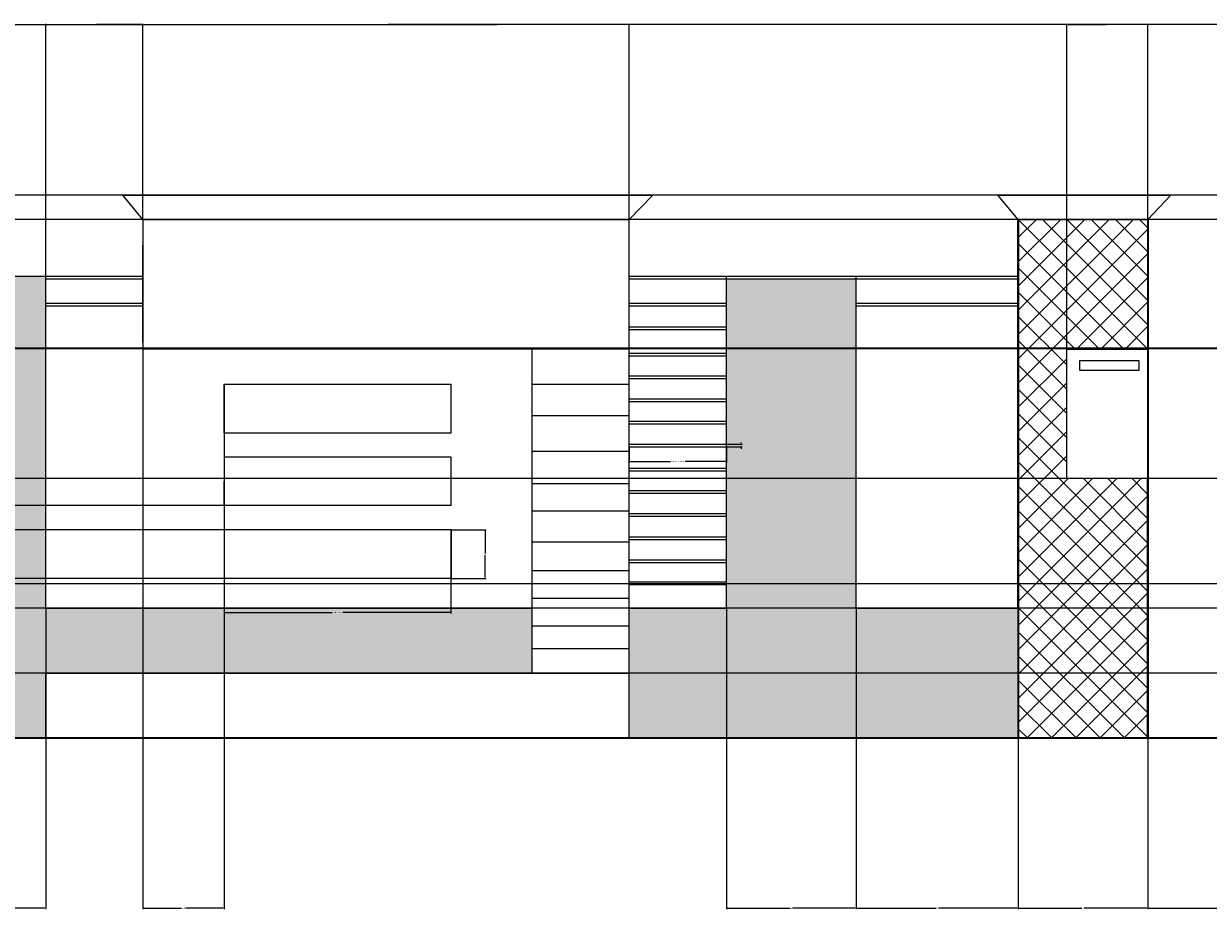
# Model space of a CAD drawing. Units: inches. Extents: x 2121 to 2815, y 1818 to 2233.
# Tile 2 of 6: x 2311 to 2530, y 1818 to 1982. Entities that reach past the tile are written whole.
import ezdxf

# ---------------------------------------------------------------- set-up
doc = ezdxf.new("R2010")
doc.units = ezdxf.units.IN
for name, color, linetype, lineweight in [('A-ANNO-DIMS', 2, 'Continuous', 18), ('A-COLS', 7, 'Continuous', 35), ('A-DETL', 7, 'Continuous', 18), ('A-ELEV', 7, 'Continuous', 25), ('A-ELEV-GRDE', 7, 'Continuous', 35), ('A-ELEV-SLAT', 7, 'Continuous', 18), ('A-WALL-COPG', 7, 'Continuous', 25), ('A-WALL-PATT', 8, 'Continuous', 13)]:
    doc.layers.add(name, color=color, linetype=linetype, lineweight=lineweight)
doc.styles.get("Standard").update_dxf_attribs({"font": 'arial.ttf'})
doc.dimstyles.get("Standard").update_dxf_attribs({"dimtxt": 0.18, "dimasz": 0.18, "dimexe": 0.18, "dimexo": 0.0625, "dimgap": 0.09, "dimtad": 0, "dimtih": 1, "dimtoh": 1, "dimdec": 4, "dimzin": 0, "dimdsep": 46, "dimtxsty": 'Standard', "dimcen": 0.09, "dimadec": 0, "dimazin": 0, "dimtfac": 1, "dimtdec": 4, "dimtofl": 0, "dimtmove": 0, "dimatfit": 3, "dimfxl": 1, "dimtolj": 1, "dimtzin": 0, "dimarcsym": 0})

# ---------------------------------------------------------------- blocks, each defined once
blk = doc.blocks.new('WALL-SLAT-18')
for p, q in [((0, 0.5), (18, 0.5)), ((0, 0), (18, 0)), ((0, 0), (18, 0))]:
    blk.add_line(p, q)
blk = doc.blocks.new('WALL-PANEL-42X9')
for p, q in [((42, 9), (0, 9)), ((0, 9), (0, 0)), ((42, 0), (42, 9)), ((42, 0), (0, 0))]:
    blk.add_line(p, q)
blk = doc.blocks.new('*D4')
at = {"layer": 'A-ANNO-DIMS', "color": 0, "lineweight": -2, "transparency": 16777216}
for p, q in [((2422.83, 1903.71), (2422.83, 1900.89)), ((2440.83, 1903.71), (2440.83, 1900.89)), ((2423.01, 1901.07), (2430.48, 1901.07)), ((2440.65, 1901.07), (2433.18, 1901.07))]:
    blk.add_line(p, q, dxfattribs=at)
at = {"layer": 'A-ANNO-DIMS', "color": 0, "transparency": 16777216}
for points in [[(2423.01, 1901.1), (2423.01, 1901.04), (2422.83, 1901.07)], [(2440.65, 1901.1), (2440.65, 1901.04), (2440.83, 1901.07)]]:
    blk.add_solid(points, dxfattribs=at)
at = {"layer": 'Defpoints', "color": 0, "transparency": 16777216}
for p in [(2422.83, 1903.77), (2440.83, 1903.77), (2440.83, 1901.07)]:
    blk.add_point(p, dxfattribs=at)
at = {"layer": 'A-ANNO-DIMS', "color": 0, "transparency": 16777216, "insert": (2431.83, 1901.07), "char_height": 0.18, "attachment_point": 5}
blk.add_mtext('\\A1;SHORT SLAT 18 TYP.', dxfattribs=at)
blk = doc.blocks.new('*D5')
at = {"layer": 'A-ANNO-DIMS', "color": 0, "lineweight": -2, "transparency": 16777216}
for p, q in [((2440.9, 1904.27), (2443.71, 1904.27)), ((2440.9, 1903.77), (2443.71, 1903.77)), ((2443.53, 1904.45), (2443.53, 1904.63)), ((2443.53, 1903.59), (2443.53, 1903.41))]:
    blk.add_line(p, q, dxfattribs=at)
at = {"layer": 'A-ANNO-DIMS', "color": 0, "transparency": 16777216}
for points in [[(2443.5, 1904.45), (2443.56, 1904.45), (2443.53, 1904.27)], [(2443.5, 1903.59), (2443.56, 1903.59), (2443.53, 1903.77)]]:
    blk.add_solid(points, dxfattribs=at)
at = {"layer": 'Defpoints', "color": 0, "transparency": 16777216}
for p in [(2440.83, 1904.27), (2440.83, 1903.77), (2443.53, 1904.27)]:
    blk.add_point(p, dxfattribs=at)
at = {"layer": 'A-ANNO-DIMS', "color": 0, "transparency": 16777216, "insert": (2443.53, 1904.02), "char_height": 0.18, "attachment_point": 5}
blk.add_mtext('\\A1;1 TYP.', dxfattribs=at)
blk = doc.blocks.new('*D6')
at = {"layer": 'A-ANNO-DIMS', "color": 0, "lineweight": -2, "transparency": 16777216}
for p, q in [((2347.83, 1879.34), (2347.83, 1872.93)), ((2389.83, 1879.34), (2389.83, 1872.93)), ((2348.01, 1873.11), (2367.86, 1873.11)), ((2389.65, 1873.11), (2369.8, 1873.11))]:
    blk.add_line(p, q, dxfattribs=at)
at = {"layer": 'A-ANNO-DIMS', "color": 0, "transparency": 16777216}
for points in [[(2348.01, 1873.14), (2348.01, 1873.08), (2347.83, 1873.11)], [(2389.65, 1873.14), (2389.65, 1873.08), (2389.83, 1873.11)]]:
    blk.add_solid(points, dxfattribs=at)
at = {"layer": 'Defpoints', "color": 0, "transparency": 16777216}
for p in [(2347.83, 1879.41), (2389.83, 1879.41), (2389.83, 1873.11)]:
    blk.add_point(p, dxfattribs=at)
at = {"layer": 'A-ANNO-DIMS', "color": 0, "transparency": 16777216, "insert": (2368.83, 1873.11), "char_height": 0.18, "attachment_point": 5}
blk.add_mtext('\\A1;PANEL 42 TYP.', dxfattribs=at)
blk = doc.blocks.new('*D7')
at = {"layer": 'A-ANNO-DIMS', "color": 0, "lineweight": -2, "transparency": 16777216}
for p, q in [((2389.9, 1888.41), (2396.31, 1888.41)), ((2396.13, 1888.23), (2396.13, 1884.09)), ((2396.13, 1879.59), (2396.13, 1883.73)), ((2389.9, 1879.41), (2396.31, 1879.41))]:
    blk.add_line(p, q, dxfattribs=at)
at = {"layer": 'A-ANNO-DIMS', "color": 0, "transparency": 16777216}
for points in [[(2396.1, 1888.23), (2396.16, 1888.23), (2396.13, 1888.41)], [(2396.1, 1879.59), (2396.16, 1879.59), (2396.13, 1879.41)]]:
    blk.add_solid(points, dxfattribs=at)
at = {"layer": 'Defpoints', "color": 0, "transparency": 16777216}
for p in [(2389.83, 1888.41), (2396.13, 1888.41), (2389.83, 1879.41)]:
    blk.add_point(p, dxfattribs=at)
at = {"layer": 'A-ANNO-DIMS', "color": 0, "transparency": 16777216, "insert": (2396.13, 1883.91), "char_height": 0.18, "attachment_point": 5}
blk.add_mtext('\\A1;9 TYP.', dxfattribs=at)
blk = doc.blocks.new('*D43')
at = {"layer": 'A-ANNO-DIMS', "color": 0, "lineweight": -2, "transparency": 16777216}
for p, q in [((2152.83, 1935.47), (2152.83, 1982.13)), ((2644.63, 1950.47), (2644.63, 1982.13)), ((2153.01, 1981.95), (2398.33, 1981.95)), ((2644.45, 1981.95), (2399.13, 1981.95))]:
    blk.add_line(p, q, dxfattribs=at)
at = {"layer": 'A-ANNO-DIMS', "color": 0, "transparency": 16777216}
for points in [[(2153.01, 1981.98), (2153.01, 1981.92), (2152.83, 1981.95)], [(2644.45, 1981.98), (2644.45, 1981.92), (2644.63, 1981.95)]]:
    blk.add_solid(points, dxfattribs=at)
at = {"layer": 'Defpoints', "color": 0, "transparency": 16777216}
for p in [(2644.63, 1981.95), (2644.63, 1950.41), (2152.83, 1935.41)]:
    blk.add_point(p, dxfattribs=at)
at = {"layer": 'A-ANNO-DIMS', "color": 0, "transparency": 16777216, "insert": (2398.73, 1981.95), "char_height": 0.18, "attachment_point": 5}
blk.add_mtext('\\A1;491.8', dxfattribs=at)
blk = doc.blocks.new('*D51')
at = {"layer": 'A-ANNO-DIMS', "color": 0, "lineweight": -2, "transparency": 16777216}
for p, q in [((2290.83, 1873.84), (2290.83, 1818.19)), ((2314.83, 1873.84), (2314.83, 1818.19)), ((2291.01, 1818.37), (2302.61, 1818.37)), ((2314.65, 1818.37), (2303.05, 1818.37))]:
    blk.add_line(p, q, dxfattribs=at)
at = {"layer": 'A-ANNO-DIMS', "color": 0, "transparency": 16777216}
for points in [[(2291.01, 1818.4), (2291.01, 1818.34), (2290.83, 1818.37)], [(2314.65, 1818.4), (2314.65, 1818.34), (2314.83, 1818.37)]]:
    blk.add_solid(points, dxfattribs=at)
at = {"layer": 'Defpoints', "color": 0, "transparency": 16777216}
for p in [(2290.83, 1873.91), (2314.83, 1873.91), (2314.83, 1818.37)]:
    blk.add_point(p, dxfattribs=at)
at = {"layer": 'A-ANNO-DIMS', "color": 0, "transparency": 16777216, "insert": (2302.83, 1818.37), "char_height": 0.18, "attachment_point": 5}
blk.add_mtext('\\A1;24', dxfattribs=at)
blk = doc.blocks.new('*D52')
at = {"layer": 'A-ANNO-DIMS', "color": 0, "lineweight": -2, "transparency": 16777216}
for p, q in [((2314.83, 1935.47), (2314.83, 1982.13)), ((2332.79, 1945.97), (2332.79, 1982.13)), ((2315.01, 1981.95), (2323.43, 1981.95)), ((2332.61, 1981.95), (2324.2, 1981.95))]:
    blk.add_line(p, q, dxfattribs=at)
at = {"layer": 'A-ANNO-DIMS', "color": 0, "transparency": 16777216}
for points in [[(2315.01, 1981.98), (2315.01, 1981.92), (2314.83, 1981.95)], [(2332.61, 1981.98), (2332.61, 1981.92), (2332.79, 1981.95)]]:
    blk.add_solid(points, dxfattribs=at)
at = {"layer": 'Defpoints', "color": 0, "transparency": 16777216}
for p in [(2332.79, 1981.95), (2332.79, 1945.91), (2314.83, 1935.41)]:
    blk.add_point(p, dxfattribs=at)
at = {"layer": 'A-ANNO-DIMS', "color": 0, "transparency": 16777216, "insert": (2323.81, 1981.95), "char_height": 0.18, "attachment_point": 5}
blk.add_mtext('\\A1;17.96', dxfattribs=at)
blk = doc.blocks.new('*D53')
at = {"layer": 'A-ANNO-DIMS', "color": 0, "lineweight": -2, "transparency": 16777216}
for p, q in [((2332.79, 1945.97), (2332.79, 1982.13)), ((2422.83, 1945.97), (2422.83, 1982.13)), ((2332.97, 1981.95), (2377.42, 1981.95)), ((2422.65, 1981.95), (2378.21, 1981.95))]:
    blk.add_line(p, q, dxfattribs=at)
at = {"layer": 'A-ANNO-DIMS', "color": 0, "transparency": 16777216}
for points in [[(2332.97, 1981.98), (2332.97, 1981.92), (2332.79, 1981.95)], [(2422.65, 1981.98), (2422.65, 1981.92), (2422.83, 1981.95)]]:
    blk.add_solid(points, dxfattribs=at)
at = {"layer": 'Defpoints', "color": 0, "transparency": 16777216}
for p in [(2422.83, 1981.95), (2332.79, 1945.91), (2422.83, 1945.91)]:
    blk.add_point(p, dxfattribs=at)
at = {"layer": 'A-ANNO-DIMS', "color": 0, "transparency": 16777216, "insert": (2377.81, 1981.95), "char_height": 0.18, "attachment_point": 5}
blk.add_mtext('\\A1;90.04', dxfattribs=at)
blk = doc.blocks.new('*D54')
at = {"layer": 'A-ANNO-DIMS', "color": 0, "lineweight": -2, "transparency": 16777216}
for p, q in [((2440.83, 1873.84), (2440.83, 1818.19)), ((2464.83, 1873.84), (2464.83, 1818.19)), ((2441.01, 1818.37), (2452.61, 1818.37)), ((2464.65, 1818.37), (2453.05, 1818.37))]:
    blk.add_line(p, q, dxfattribs=at)
at = {"layer": 'A-ANNO-DIMS', "color": 0, "transparency": 16777216}
for points in [[(2441.01, 1818.4), (2441.01, 1818.34), (2440.83, 1818.37)], [(2464.65, 1818.4), (2464.65, 1818.34), (2464.83, 1818.37)]]:
    blk.add_solid(points, dxfattribs=at)
at = {"layer": 'Defpoints', "color": 0, "transparency": 16777216}
for p in [(2440.83, 1873.91), (2464.83, 1873.91), (2464.83, 1818.37)]:
    blk.add_point(p, dxfattribs=at)
at = {"layer": 'A-ANNO-DIMS', "color": 0, "transparency": 16777216, "insert": (2452.83, 1818.37), "char_height": 0.18, "attachment_point": 5}
blk.add_mtext('\\A1;24', dxfattribs=at)
blk = doc.blocks.new('*D55')
at = {"layer": 'A-ANNO-DIMS', "color": 0, "lineweight": -2, "transparency": 16777216}
for p, q in [((2464.83, 1873.84), (2464.83, 1818.19)), ((2494.83, 1873.84), (2494.83, 1818.19)), ((2465.01, 1818.37), (2479.61, 1818.37)), ((2494.65, 1818.37), (2480.05, 1818.37))]:
    blk.add_line(p, q, dxfattribs=at)
at = {"layer": 'A-ANNO-DIMS', "color": 0, "transparency": 16777216}
for points in [[(2465.01, 1818.4), (2465.01, 1818.34), (2464.83, 1818.37)], [(2494.65, 1818.4), (2494.65, 1818.34), (2494.83, 1818.37)]]:
    blk.add_solid(points, dxfattribs=at)
at = {"layer": 'Defpoints', "color": 0, "transparency": 16777216}
for p in [(2464.83, 1873.91), (2494.83, 1873.91), (2494.83, 1818.37)]:
    blk.add_point(p, dxfattribs=at)
at = {"layer": 'A-ANNO-DIMS', "color": 0, "transparency": 16777216, "insert": (2479.83, 1818.37), "char_height": 0.18, "attachment_point": 5}
blk.add_mtext('\\A1;30', dxfattribs=at)
blk = doc.blocks.new('*D56')
at = {"layer": 'A-ANNO-DIMS', "color": 0, "lineweight": -2, "transparency": 16777216}
for p, q in [((2494.83, 1849.84), (2494.83, 1818.19)), ((2518.83, 1849.84), (2518.83, 1818.19)), ((2495.01, 1818.37), (2506.61, 1818.37)), ((2518.65, 1818.37), (2507.05, 1818.37))]:
    blk.add_line(p, q, dxfattribs=at)
at = {"layer": 'A-ANNO-DIMS', "color": 0, "transparency": 16777216}
for points in [[(2495.01, 1818.4), (2495.01, 1818.34), (2494.83, 1818.37)], [(2518.65, 1818.4), (2518.65, 1818.34), (2518.83, 1818.37)]]:
    blk.add_solid(points, dxfattribs=at)
at = {"layer": 'Defpoints', "color": 0, "transparency": 16777216}
for p in [(2494.83, 1849.91), (2518.83, 1849.91), (2518.83, 1818.37)]:
    blk.add_point(p, dxfattribs=at)
at = {"layer": 'A-ANNO-DIMS', "color": 0, "transparency": 16777216, "insert": (2506.83, 1818.37), "char_height": 0.18, "attachment_point": 5}
blk.add_mtext('\\A1;24', dxfattribs=at)
blk = doc.blocks.new('*D57')
at = {"layer": 'A-ANNO-DIMS', "color": 0, "lineweight": -2, "transparency": 16777216}
for p, q in [((2518.83, 1849.84), (2518.83, 1818.19)), ((2619.83, 1849.84), (2619.83, 1818.19)), ((2519.01, 1818.37), (2569.07, 1818.37)), ((2619.65, 1818.37), (2569.6, 1818.37))]:
    blk.add_line(p, q, dxfattribs=at)
at = {"layer": 'A-ANNO-DIMS', "color": 0, "transparency": 16777216}
for points in [[(2519.01, 1818.4), (2519.01, 1818.34), (2518.83, 1818.37)], [(2619.65, 1818.4), (2619.65, 1818.34), (2619.83, 1818.37)]]:
    blk.add_solid(points, dxfattribs=at)
at = {"layer": 'Defpoints', "color": 0, "transparency": 16777216}
for p in [(2518.83, 1849.91), (2619.83, 1849.91), (2619.83, 1818.37)]:
    blk.add_point(p, dxfattribs=at)
at = {"layer": 'A-ANNO-DIMS', "color": 0, "transparency": 16777216, "insert": (2569.33, 1818.37), "char_height": 0.18, "attachment_point": 5}
blk.add_mtext('\\A1;101', dxfattribs=at)
blk = doc.blocks.new('*D59')
at = {"layer": 'A-ANNO-DIMS', "color": 0, "lineweight": -2, "transparency": 16777216}
for p, q in [((2182.9, 1922.1), (2815, 1922.1)), ((2814.82, 1921.92), (2814.82, 1886.18)), ((2814.82, 1850.09), (2814.82, 1885.82)), ((2182.9, 1849.91), (2815, 1849.91))]:
    blk.add_line(p, q, dxfattribs=at)
at = {"layer": 'A-ANNO-DIMS', "color": 0, "transparency": 16777216}
for points in [[(2814.79, 1921.92), (2814.85, 1921.92), (2814.82, 1922.1)], [(2814.79, 1850.09), (2814.85, 1850.09), (2814.82, 1849.91)]]:
    blk.add_solid(points, dxfattribs=at)
at = {"layer": 'Defpoints', "color": 0, "transparency": 16777216}
for p in [(2182.83, 1922.1), (2814.82, 1922.1), (2182.83, 1849.91)]:
    blk.add_point(p, dxfattribs=at)
at = {"layer": 'A-ANNO-DIMS', "color": 0, "transparency": 16777216, "insert": (2814.82, 1886), "char_height": 0.18, "attachment_point": 5}
blk.add_mtext('\\A1;72.2', dxfattribs=at)
blk = doc.blocks.new('*D61')
at = {"layer": 'A-ANNO-DIMS', "color": 0, "lineweight": -2, "transparency": 16777216}
for p, q in [((2314.77, 1861.91), (2121.11, 1861.91)), ((2121.29, 1861.73), (2121.29, 1856.09)), ((2121.29, 1850.09), (2121.29, 1855.73)), ((2314.77, 1849.91), (2121.11, 1849.91))]:
    blk.add_line(p, q, dxfattribs=at)
at = {"layer": 'A-ANNO-DIMS', "color": 0, "transparency": 16777216}
for points in [[(2121.26, 1861.73), (2121.32, 1861.73), (2121.29, 1861.91)], [(2121.26, 1850.09), (2121.32, 1850.09), (2121.29, 1849.91)]]:
    blk.add_solid(points, dxfattribs=at)
at = {"layer": 'Defpoints', "color": 0, "transparency": 16777216}
for p in [(2121.29, 1861.91), (2314.83, 1861.91), (2314.83, 1849.91)]:
    blk.add_point(p, dxfattribs=at)
at = {"layer": 'A-ANNO-DIMS', "color": 0, "transparency": 16777216, "insert": (2121.29, 1855.91), "char_height": 0.18, "attachment_point": 5}
blk.add_mtext('\\A1;12', dxfattribs=at)
blk = doc.blocks.new('*D62')
at = {"layer": 'A-ANNO-DIMS', "color": 0, "lineweight": -2, "transparency": 16777216}
for p, q in [((2332.79, 1921.84), (2332.79, 1818.19)), ((2347.83, 1915.34), (2347.83, 1818.19)), ((2332.97, 1818.37), (2339.93, 1818.37)), ((2347.65, 1818.37), (2340.7, 1818.37))]:
    blk.add_line(p, q, dxfattribs=at)
at = {"layer": 'A-ANNO-DIMS', "color": 0, "transparency": 16777216}
for points in [[(2332.97, 1818.4), (2332.97, 1818.34), (2332.79, 1818.37)], [(2347.65, 1818.4), (2347.65, 1818.34), (2347.83, 1818.37)]]:
    blk.add_solid(points, dxfattribs=at)
at = {"layer": 'Defpoints', "color": 0, "transparency": 16777216}
for p in [(2332.79, 1921.91), (2347.83, 1915.41), (2347.83, 1818.37)]:
    blk.add_point(p, dxfattribs=at)
at = {"layer": 'A-ANNO-DIMS', "color": 0, "transparency": 16777216, "insert": (2340.31, 1818.37), "char_height": 0.18, "attachment_point": 5}
blk.add_mtext('\\A1;15.04', dxfattribs=at)
blk = doc.blocks.new('*D63')
at = {"layer": 'A-ANNO-DIMS', "color": 0, "lineweight": -2, "transparency": 16777216}
for p, q in [((2347.77, 1892.91), (2121.11, 1892.91)), ((2121.29, 1892.73), (2121.29, 1890.84)), ((2121.29, 1888.59), (2121.29, 1890.48)), ((2347.77, 1888.41), (2121.11, 1888.41))]:
    blk.add_line(p, q, dxfattribs=at)
at = {"layer": 'A-ANNO-DIMS', "color": 0, "transparency": 16777216}
for points in [[(2121.26, 1892.73), (2121.32, 1892.73), (2121.29, 1892.91)], [(2121.26, 1888.59), (2121.32, 1888.59), (2121.29, 1888.41)]]:
    blk.add_solid(points, dxfattribs=at)
at = {"layer": 'Defpoints', "color": 0, "transparency": 16777216}
for p in [(2121.29, 1892.91), (2347.83, 1892.91), (2347.83, 1888.41)]:
    blk.add_point(p, dxfattribs=at)
at = {"layer": 'A-ANNO-DIMS', "color": 0, "transparency": 16777216, "insert": (2121.29, 1890.66), "char_height": 0.18, "attachment_point": 5}
blk.add_mtext('\\A1;4.5', dxfattribs=at)
blk = doc.blocks.new('*D64')
at = {"layer": 'A-ANNO-DIMS', "color": 0, "lineweight": -2, "transparency": 16777216}
for p, q in [((2347.77, 1879.41), (2121.11, 1879.41)), ((2121.29, 1879.23), (2121.29, 1876.84)), ((2121.29, 1874.09), (2121.29, 1876.48)), ((2314.77, 1873.91), (2121.11, 1873.91))]:
    blk.add_line(p, q, dxfattribs=at)
at = {"layer": 'A-ANNO-DIMS', "color": 0, "transparency": 16777216}
for points in [[(2121.26, 1879.23), (2121.32, 1879.23), (2121.29, 1879.41)], [(2121.26, 1874.09), (2121.32, 1874.09), (2121.29, 1873.91)]]:
    blk.add_solid(points, dxfattribs=at)
at = {"layer": 'Defpoints', "color": 0, "transparency": 16777216}
for p in [(2121.29, 1879.41), (2347.83, 1879.41), (2314.83, 1873.91)]:
    blk.add_point(p, dxfattribs=at)
at = {"layer": 'A-ANNO-DIMS', "color": 0, "transparency": 16777216, "insert": (2121.29, 1876.66), "char_height": 0.18, "attachment_point": 5}
blk.add_mtext('\\A1;5.5', dxfattribs=at)
blk = doc.blocks.new('*D65')
at = {"layer": 'A-ANNO-DIMS', "color": 0, "lineweight": -2, "transparency": 16777216}
for p, q in [((2619.77, 1897.91), (2121.11, 1897.91)), ((2121.29, 1897.73), (2121.29, 1874.09)), ((2121.29, 1850.09), (2121.29, 1873.73)), ((2619.77, 1849.91), (2121.11, 1849.91))]:
    blk.add_line(p, q, dxfattribs=at)
at = {"layer": 'A-ANNO-DIMS', "color": 0, "transparency": 16777216}
for points in [[(2121.26, 1897.73), (2121.32, 1897.73), (2121.29, 1897.91)], [(2121.26, 1850.09), (2121.32, 1850.09), (2121.29, 1849.91)]]:
    blk.add_solid(points, dxfattribs=at)
at = {"layer": 'Defpoints', "color": 0, "transparency": 16777216}
for p in [(2121.29, 1897.91), (2619.83, 1897.91), (2619.83, 1849.91)]:
    blk.add_point(p, dxfattribs=at)
at = {"layer": 'A-ANNO-DIMS', "color": 0, "transparency": 16777216, "insert": (2121.29, 1873.91), "char_height": 0.18, "attachment_point": 5}
blk.add_mtext('\\A1;48', dxfattribs=at)
blk = doc.blocks.new('*D66')
at = {"layer": 'A-ANNO-DIMS', "color": 0, "lineweight": -2, "transparency": 16777216}
for p, q in [((2619.77, 1921.91), (2121.11, 1921.91)), ((2121.29, 1921.73), (2121.29, 1910.09)), ((2121.29, 1898.09), (2121.29, 1909.73)), ((2619.77, 1897.91), (2121.11, 1897.91))]:
    blk.add_line(p, q, dxfattribs=at)
at = {"layer": 'A-ANNO-DIMS', "color": 0, "transparency": 16777216}
for points in [[(2121.26, 1921.73), (2121.32, 1921.73), (2121.29, 1921.91)], [(2121.26, 1898.09), (2121.32, 1898.09), (2121.29, 1897.91)]]:
    blk.add_solid(points, dxfattribs=at)
at = {"layer": 'Defpoints', "color": 0, "transparency": 16777216}
for p in [(2121.29, 1921.91), (2619.83, 1921.91), (2619.83, 1897.91)]:
    blk.add_point(p, dxfattribs=at)
at = {"layer": 'A-ANNO-DIMS', "color": 0, "transparency": 16777216, "insert": (2121.29, 1909.91), "char_height": 0.18, "attachment_point": 5}
blk.add_mtext('\\A1;24', dxfattribs=at)
blk = doc.blocks.new('*D68')
at = {"layer": 'A-ANNO-DIMS', "color": 0, "lineweight": -2, "transparency": 16777216}
for p, q in [((2503.83, 1921.97), (2503.83, 1982.13)), ((2518.83, 1921.97), (2518.83, 1982.13)), ((2504.01, 1981.95), (2511.12, 1981.95)), ((2518.65, 1981.95), (2511.54, 1981.95))]:
    blk.add_line(p, q, dxfattribs=at)
at = {"layer": 'A-ANNO-DIMS', "color": 0, "transparency": 16777216}
for points in [[(2504.01, 1981.98), (2504.01, 1981.92), (2503.83, 1981.95)], [(2518.65, 1981.98), (2518.65, 1981.92), (2518.83, 1981.95)]]:
    blk.add_solid(points, dxfattribs=at)
at = {"layer": 'Defpoints', "color": 0, "transparency": 16777216}
for p in [(2518.83, 1981.95), (2503.83, 1921.91), (2518.83, 1921.91)]:
    blk.add_point(p, dxfattribs=at)
at = {"layer": 'A-ANNO-DIMS', "color": 0, "transparency": 16777216, "insert": (2511.33, 1981.95), "char_height": 0.18, "attachment_point": 5}
blk.add_mtext('\\A1;15', dxfattribs=at)
blk = doc.blocks.new('*D72')
at = {"layer": 'A-ANNO-DIMS', "color": 0, "lineweight": -2, "transparency": 16777216}
for p, q in [((2760.77, 1861.91), (2121.11, 1861.91)), ((2121.29, 1861.73), (2121.29, 1856.09)), ((2121.29, 1850.09), (2121.29, 1855.73)), ((2760.77, 1849.91), (2121.11, 1849.91))]:
    blk.add_line(p, q, dxfattribs=at)
at = {"layer": 'A-ANNO-DIMS', "color": 0, "transparency": 16777216}
for points in [[(2121.26, 1861.73), (2121.32, 1861.73), (2121.29, 1861.91)], [(2121.26, 1850.09), (2121.32, 1850.09), (2121.29, 1849.91)]]:
    blk.add_solid(points, dxfattribs=at)
at = {"layer": 'Defpoints', "color": 0, "transparency": 16777216}
for p in [(2121.29, 1861.91), (2760.83, 1861.91), (2760.83, 1849.91)]:
    blk.add_point(p, dxfattribs=at)
at = {"layer": 'A-ANNO-DIMS', "color": 0, "transparency": 16777216, "insert": (2121.29, 1855.91), "char_height": 0.18, "attachment_point": 5}
blk.add_mtext('\\A1;12', dxfattribs=at)
blk = doc.blocks.new('*D73')
at = {"layer": 'A-ANNO-DIMS', "color": 0, "lineweight": -2, "transparency": 16777216}
for p, q in [((2765.27, 1873.91), (2121.11, 1873.91)), ((2121.29, 1873.73), (2121.29, 1868.09)), ((2121.29, 1862.09), (2121.29, 1867.73)), ((2760.77, 1861.91), (2121.11, 1861.91))]:
    blk.add_line(p, q, dxfattribs=at)
at = {"layer": 'A-ANNO-DIMS', "color": 0, "transparency": 16777216}
for points in [[(2121.26, 1873.73), (2121.32, 1873.73), (2121.29, 1873.91)], [(2121.26, 1862.09), (2121.32, 1862.09), (2121.29, 1861.91)]]:
    blk.add_solid(points, dxfattribs=at)
at = {"layer": 'Defpoints', "color": 0, "transparency": 16777216}
for p in [(2121.29, 1873.91), (2765.33, 1873.91), (2760.83, 1861.91)]:
    blk.add_point(p, dxfattribs=at)
at = {"layer": 'A-ANNO-DIMS', "color": 0, "transparency": 16777216, "insert": (2121.29, 1867.91), "char_height": 0.18, "attachment_point": 5}
blk.add_mtext('\\A1;12', dxfattribs=at)
blk = doc.blocks.new('*D74')
at = {"layer": 'A-ANNO-DIMS', "color": 0, "lineweight": -2, "transparency": 16777216}
for p, q in [((2765.27, 1921.91), (2121.11, 1921.91)), ((2121.29, 1921.73), (2121.29, 1898.09)), ((2121.29, 1874.09), (2121.29, 1897.73)), ((2765.27, 1873.91), (2121.11, 1873.91))]:
    blk.add_line(p, q, dxfattribs=at)
at = {"layer": 'A-ANNO-DIMS', "color": 0, "transparency": 16777216}
for points in [[(2121.26, 1921.73), (2121.32, 1921.73), (2121.29, 1921.91)], [(2121.26, 1874.09), (2121.32, 1874.09), (2121.29, 1873.91)]]:
    blk.add_solid(points, dxfattribs=at)
at = {"layer": 'Defpoints', "color": 0, "transparency": 16777216}
for p in [(2121.29, 1921.91), (2765.33, 1921.91), (2765.33, 1873.91)]:
    blk.add_point(p, dxfattribs=at)
at = {"layer": 'A-ANNO-DIMS', "color": 0, "transparency": 16777216, "insert": (2121.29, 1897.91), "char_height": 0.18, "attachment_point": 5}
blk.add_mtext('\\A1;48', dxfattribs=at)
blk = doc.blocks.new('*D75')
at = {"layer": 'A-ANNO-DIMS', "color": 0, "lineweight": -2, "transparency": 16777216}
for p, q in [((2760.77, 1945.91), (2121.11, 1945.91)), ((2121.29, 1945.73), (2121.29, 1934.09)), ((2121.29, 1922.09), (2121.29, 1933.73)), ((2760.77, 1921.91), (2121.11, 1921.91))]:
    blk.add_line(p, q, dxfattribs=at)
at = {"layer": 'A-ANNO-DIMS', "color": 0, "transparency": 16777216}
for points in [[(2121.26, 1945.73), (2121.32, 1945.73), (2121.29, 1945.91)], [(2121.26, 1922.09), (2121.32, 1922.09), (2121.29, 1921.91)]]:
    blk.add_solid(points, dxfattribs=at)
at = {"layer": 'Defpoints', "color": 0, "transparency": 16777216}
for p in [(2121.29, 1945.91), (2760.83, 1945.91), (2760.83, 1921.91)]:
    blk.add_point(p, dxfattribs=at)
at = {"layer": 'A-ANNO-DIMS', "color": 0, "transparency": 16777216, "insert": (2121.29, 1933.91), "char_height": 0.18, "attachment_point": 5}
blk.add_mtext('\\A1;24', dxfattribs=at)
blk = doc.blocks.new('*D76')
at = {"layer": 'A-ANNO-DIMS', "color": 0, "lineweight": -2, "transparency": 16777216}
for p, q in [((2756.87, 1950.41), (2121.11, 1950.41)), ((2121.29, 1950.23), (2121.29, 1948.34)), ((2121.29, 1946.09), (2121.29, 1947.98)), ((2760.77, 1945.91), (2121.11, 1945.91))]:
    blk.add_line(p, q, dxfattribs=at)
at = {"layer": 'A-ANNO-DIMS', "color": 0, "transparency": 16777216}
for points in [[(2121.26, 1950.23), (2121.32, 1950.23), (2121.29, 1950.41)], [(2121.26, 1946.09), (2121.32, 1946.09), (2121.29, 1945.91)]]:
    blk.add_solid(points, dxfattribs=at)
at = {"layer": 'Defpoints', "color": 0, "transparency": 16777216}
for p in [(2121.29, 1950.41), (2756.93, 1950.41), (2760.83, 1945.91)]:
    blk.add_point(p, dxfattribs=at)
at = {"layer": 'A-ANNO-DIMS', "color": 0, "transparency": 16777216, "insert": (2121.29, 1948.16), "char_height": 0.18, "attachment_point": 5}
blk.add_mtext('\\A1;4.5', dxfattribs=at)
blk = doc.blocks.new('*D82')
at = {"layer": 'A-ANNO-DIMS', "color": 0, "lineweight": -2, "transparency": 16777216}
for p, q in [((2769.77, 1878.41), (2121.11, 1878.41)), ((2121.29, 1878.23), (2121.29, 1876.34)), ((2121.29, 1874.09), (2121.29, 1875.98)), ((2769.77, 1873.91), (2121.11, 1873.91))]:
    blk.add_line(p, q, dxfattribs=at)
at = {"layer": 'A-ANNO-DIMS', "color": 0, "transparency": 16777216}
for points in [[(2121.26, 1878.23), (2121.32, 1878.23), (2121.29, 1878.41)], [(2121.26, 1874.09), (2121.32, 1874.09), (2121.29, 1873.91)]]:
    blk.add_solid(points, dxfattribs=at)
at = {"layer": 'Defpoints', "color": 0, "transparency": 16777216}
for p in [(2121.29, 1878.41), (2769.83, 1878.41), (2769.83, 1873.91)]:
    blk.add_point(p, dxfattribs=at)
at = {"layer": 'A-ANNO-DIMS', "color": 0, "transparency": 16777216, "insert": (2121.29, 1876.16), "char_height": 0.18, "attachment_point": 5}
blk.add_mtext('\\A1;4.5', dxfattribs=at)

msp = doc.modelspace()

# ---------------------------------------------------------------- hatches: boundary and pattern name
at = {"layer": 'A-WALL-PATT'}
h = msp.add_hatch(dxfattribs=at)
h.set_pattern_fill('ANSI37', color=256)
h.paths.add_polyline_path([(2518.8326, 1945.9075), (2494.8326, 1945.9075), (2494.8326, 1849.9075), (2503.8326, 1849.9075), (2518.8326, 1849.9075), (2518.8326, 1897.9075), (2503.8326, 1897.9075), (2503.8326, 1921.9075), (2518.8326, 1921.9075)])
h.paths.add_polyline_path([(2640.8326, 1945.9075), (2619.8326, 1945.9075), (2619.8326, 1921.9075), (2628.8326, 1921.9075), (2628.8326, 1897.9075), (2619.8326, 1897.9075), (2619.8326, 1849.9075), (2640.8326, 1849.9075)])
h = msp.add_hatch(dxfattribs=at)
h.set_pattern_fill('DOTS', color=256)
h.paths.add_polyline_path([(2182.8326, 1873.9075), (2152.8326, 1873.9075), (2152.8326, 1849.9075), (2182.8326, 1849.9075)])
h.paths.add_polyline_path([(2404.8326, 1873.9075), (2314.8326, 1873.9075), (2314.8326, 1935.4075), (2290.8326, 1935.4075), (2290.8326, 1873.9075), (2272.8326, 1873.9075), (2224.8326, 1873.9075), (2224.8326, 1849.9075), (2314.8326, 1849.9075), (2314.8326, 1861.9075), (2404.8326, 1861.9075)])
h.paths.add_polyline_path([(2464.8326, 1934.9075), (2440.8326, 1934.9075), (2440.8326, 1873.9075), (2422.8326, 1873.9075), (2422.8326, 1849.9075), (2440.8326, 1849.9075), (2464.8326, 1849.9075), (2494.8326, 1849.9075), (2494.8326, 1873.9075), (2464.8326, 1873.9075)])

# ---------------------------------------------------------------- linework, layer by layer
at = {"layer": 'A-COLS'}
for p, q in [((2494.8326, 1873.9075), (2494.8326, 1945.9075)), ((2494.8326, 1945.9075), (2494.8326, 1849.9075)), ((2518.8326, 1945.9075), (2518.8326, 1849.9075)), ((2518.8326, 1849.9075), (2518.8326, 1897.9075))]:
    msp.add_line(p, q, dxfattribs=at)
at = {"layer": 'A-DETL'}
for p, q in [((2503.8326, 1897.9075), (2503.8326, 1921.9075)), ((2503.8326, 1897.9075), (2503.8326, 1921.9075)), ((2503.8326, 1897.9075), (2503.8326, 1921.9075)), ((2503.8326, 1921.9075), (2518.8326, 1921.9075)), ((2506.2169, 1919.7599), (2517.1316, 1919.7599)), ((2506.2169, 1917.9106), (2506.2169, 1919.7599)), ((2517.1316, 1919.7599), (2517.1316, 1917.9106)), ((2517.1316, 1917.9106), (2506.2169, 1917.9106)), ((2347.8326, 1906.4075), (2347.8326, 1915.4075)), ((2389.8326, 1906.4075), (2389.8326, 1915.4075)), ((2422.8326, 1915.3533), (2404.8326, 1915.3533)), ((2422.8326, 1909.5628), (2404.8326, 1909.5628)), ((2347.8326, 1901.9075), (2347.8326, 1892.9075)), ((2389.8326, 1892.9075), (2389.8326, 1901.9075)), ((2422.8326, 1902.9207), (2404.8326, 1902.9207)), ((2347.8326, 1892.9075), (2347.8326, 1897.4075)), ((2422.8326, 1896.9478), (2404.8326, 1896.9478)), ((2518.8326, 1897.9075), (2503.8326, 1897.9075)), ((2422.8326, 1891.8713), (2404.8326, 1891.8713)), ((2389.8326, 1879.4075), (2389.8326, 1888.4075)), ((2389.8326, 1888.4075), (2389.8326, 1879.4075)), ((2422.8326, 1886.132), (2404.8326, 1886.132)), ((2422.8326, 1880.828), (2404.8326, 1880.828)), ((2422.8326, 1875.7303), (2404.8326, 1875.7303)), ((2422.8326, 1870.5748), (2404.8326, 1870.5748)), ((2422.8326, 1866.404), (2404.8326, 1866.404))]:
    msp.add_line(p, q, dxfattribs=at)
at = {"layer": 'A-ELEV'}
for p, q in [((2332.7939, 1945.9075), (2332.7939, 1921.9075)), ((2422.8326, 1849.9075), (2422.8326, 1945.9075)), ((2332.7939, 1923.0879), (2332.7939, 1941.1047)), ((2314.8326, 1873.9075), (2314.8326, 1935.4075)), ((2440.8326, 1873.9075), (2440.8326, 1935.4075)), ((2464.8326, 1873.9075), (2464.8326, 1935.4075)), ((2422.8326, 1921.9075), (2332.7939, 1921.9075)), ((2389.8326, 1921.9075), (2347.8326, 1921.9075)), ((2404.8326, 1921.9075), (2389.8326, 1921.9075)), ((2404.8326, 1861.9075), (2404.8326, 1921.9075)), ((2404.8326, 1873.9075), (2404.8326, 1921.9075)), ((2314.8326, 1873.9075), (2404.8326, 1873.9075)), ((2440.8326, 1873.9075), (2422.8326, 1873.9075)), ((2422.8326, 1873.9075), (2440.8326, 1873.9075)), ((2464.8326, 1873.9075), (2494.8326, 1873.9075)), ((2464.8326, 1873.9075), (2494.8326, 1873.9075)), ((2314.8326, 1861.9075), (2314.8326, 1849.9075)), ((2314.8326, 1849.9075), (2314.8326, 1861.9075)), ((2314.8326, 1861.9075), (2422.8326, 1861.9075))]:
    msp.add_line(p, q, dxfattribs=at)
at = {"layer": 'A-ELEV-GRDE'}
for p, q in [((2152.8326, 1849.9075), (2778.8326, 1849.9075)), ((2314.8326, 1849.9075), (2347.8326, 1849.9075)), ((2347.8326, 1849.9075), (2389.8326, 1849.9075)), ((2389.8326, 1849.9075), (2404.8326, 1849.9075)), ((2404.8326, 1849.9075), (2422.8326, 1849.9075)), ((2422.8326, 1849.9075), (2440.8326, 1849.9075)), ((2440.8326, 1849.9075), (2464.8326, 1849.9075)), ((2494.8326, 1849.9075), (2503.8326, 1849.9075)), ((2518.8326, 1849.9075), (2619.8326, 1849.9075))]:
    msp.add_line(p, q, dxfattribs=at)
at = {"layer": 'A-ELEV-SLAT'}
for p, q in [((2272.8326, 1935.4075), (2332.7939, 1935.4075)), ((2314.8326, 1934.9075), (2332.7939, 1934.9075)), ((2422.8326, 1935.4075), (2494.8326, 1935.4075)), ((2422.8326, 1934.9075), (2494.8326, 1934.9075)), ((2314.8326, 1930.4075), (2332.7939, 1930.4075)), ((2314.8326, 1929.9075), (2332.7939, 1929.9075)), ((2464.8326, 1930.4075), (2494.8326, 1930.4075)), ((2464.8326, 1929.9075), (2494.8326, 1929.9075))]:
    msp.add_line(p, q, dxfattribs=at)
at = {"layer": 'A-WALL-COPG'}
for p, q in [((2332.7939, 1945.9075), (2329.0976, 1950.4075)), ((2329.0976, 1950.4075), (2427.2083, 1950.4075)), ((2422.8326, 1945.9075), (2427.2083, 1950.4075)), ((2494.8326, 1945.9075), (2491.0184, 1950.4075)), ((2491.0184, 1950.4075), (2523.0578, 1950.4075)), ((2518.8326, 1945.9075), (2523.0578, 1950.4075)), ((2332.7939, 1945.9075), (2422.8326, 1945.9075)), ((2494.8326, 1945.9075), (2518.8326, 1945.9075)), ((2503.8326, 1945.9075), (2518.8326, 1945.9075))]:
    msp.add_line(p, q, dxfattribs=at)

# ---------------------------------------------------------------- block references
at = {"layer": 'A-DETL', "rotation": 180}
msp.add_blockref('WALL-PANEL-42X9', (2389.8326, 1915.4075), dxfattribs=at)
at = {"layer": 'A-DETL'}
for p in [(2347.8326, 1892.9075), (2347.8326, 1879.4075)]:
    msp.add_blockref('WALL-PANEL-42X9', p, dxfattribs=at)
at = {"layer": 'A-ELEV-SLAT'}
for p in [(2422.8326, 1929.9075), (2422.8326, 1925.5167), (2422.8326, 1920.655), (2422.8326, 1916.4235), (2422.8326, 1912.192), (2422.8326, 1908.0505), (2422.8326, 1903.7676), (2422.8326, 1899.3444), (2422.8326, 1895.1921), (2422.8326, 1890.9494), (2422.8326, 1886.6165), (2422.8326, 1882.3738), (2422.8326, 1878.3117)]:
    msp.add_blockref('WALL-SLAT-18', p, dxfattribs=at)

# ---------------------------------------------------------------- dimensions: what is measured, and where the dimension line sits
at = {"layer": 'A-ANNO-DIMS'}
for base, p1, p2, override, picture, middle in [((2644.6318, 1981.9475), (2152.8326, 1935.4075), (2644.6318, 1950.4075), {"dimdec": 1, "dimlfac": 1, "dimrnd": 0, "dimzin": 0, "dimdsep": 46, "dimlunit": 2}, '*D43', (2398.7322, 1981.9475)), ((2332.7939, 1981.9475), (2314.8326, 1935.4075), (2332.7939, 1945.9075), {"dimdec": 2, "dimlfac": 1, "dimrnd": 0, "dimzin": 0, "dimdsep": 46, "dimlunit": 2}, '*D52', (2323.8133, 1981.9475)), ((2422.8326, 1981.9475), (2332.7939, 1945.9075), (2422.8326, 1945.9075), {"dimdec": 2, "dimlfac": 1, "dimrnd": 0, "dimzin": 0, "dimdsep": 46, "dimlunit": 2}, '*D53', (2377.8133, 1981.9475)), ((2518.8326, 1981.9475), (2503.8326, 1921.9075), (2518.8326, 1921.9075), {"dimdec": 0, "dimlfac": 1, "dimrnd": 0, "dimzin": 0, "dimdsep": 46, "dimlunit": 2}, '*D68', (2511.3326, 1981.9475)), ((2347.8326, 1818.3675), (2332.7939, 1921.9075), (2347.8326, 1915.4075), {"dimdec": 2, "dimlfac": 1, "dimrnd": 0, "dimzin": 0, "dimdsep": 46, "dimlunit": 2}, '*D62', (2340.3133, 1818.3675)), ((2314.8326, 1818.3675), (2290.8326, 1873.9075), (2314.8326, 1873.9075), {"dimdec": 0, "dimlfac": 1, "dimrnd": 0, "dimzin": 0, "dimdsep": 46, "dimlunit": 2}, '*D51', (2302.8326, 1818.3675)), ((2464.8326, 1818.3675), (2440.8326, 1873.9075), (2464.8326, 1873.9075), {"dimdec": 0, "dimlfac": 1, "dimrnd": 0, "dimzin": 0, "dimdsep": 46, "dimlunit": 2}, '*D54', (2452.8326, 1818.3675)), ((2494.8326, 1818.3675), (2464.8326, 1873.9075), (2494.8326, 1873.9075), {"dimdec": 0, "dimlfac": 1, "dimrnd": 0, "dimzin": 0, "dimdsep": 46, "dimlunit": 2}, '*D55', (2479.8326, 1818.3675)), ((2518.8326, 1818.3675), (2494.8326, 1849.9075), (2518.8326, 1849.9075), {"dimdec": 0, "dimlfac": 1, "dimrnd": 0, "dimzin": 0, "dimdsep": 46, "dimlunit": 2}, '*D56', (2506.8326, 1818.3675)), ((2619.8326, 1818.3675), (2518.8326, 1849.9075), (2619.8326, 1849.9075), {"dimdec": 0, "dimlfac": 1, "dimrnd": 0, "dimzin": 0, "dimdsep": 46, "dimlunit": 2}, '*D57', (2569.3326, 1818.3675))]:
    dim = msp.add_linear_dim(base=base, p1=p1, p2=p2, dimstyle='Standard', override=override, dxfattribs=at)
    dim.commit()
    dim.dimension.update_dxf_attribs({"geometry": picture, "text_midpoint": middle})
for base, p1, p2, override, picture, middle in [((2121.2926, 1950.4075), (2760.8326, 1945.9075), (2756.9306, 1950.4075), {"dimdec": 1, "dimlfac": 1, "dimrnd": 0, "dimzin": 0, "dimdsep": 46, "dimlunit": 2}, '*D76', (2121.2926, 1948.1575)), ((2121.2926, 1945.9075), (2760.8326, 1921.9075), (2760.8326, 1945.9075), {"dimdec": 0, "dimlfac": 1, "dimrnd": 0, "dimzin": 0, "dimdsep": 46, "dimlunit": 2}, '*D75', (2121.2926, 1933.9075)), ((2121.2926, 1921.9075), (2619.8326, 1897.9075), (2619.8326, 1921.9075), {"dimdec": 0, "dimlfac": 1, "dimrnd": 0, "dimzin": 0, "dimdsep": 46, "dimlunit": 2}, '*D66', (2121.2926, 1909.9075)), ((2121.2926, 1921.9075), (2765.3326, 1873.9075), (2765.3326, 1921.9075), {"dimdec": 0, "dimlfac": 1, "dimrnd": 0, "dimzin": 0, "dimdsep": 46, "dimlunit": 2}, '*D74', (2121.2926, 1897.9075)), ((2814.82, 1922.1005), (2182.8326, 1849.9075), (2182.8326, 1922.1005), {"dimdec": 1, "dimlfac": 1, "dimrnd": 0, "dimzin": 0, "dimdsep": 46, "dimlunit": 2}, '*D59', (2814.82, 1886.004)), ((2121.2926, 1897.9075), (2619.8326, 1849.9075), (2619.8326, 1897.9075), {"dimdec": 0, "dimlfac": 1, "dimrnd": 0, "dimzin": 0, "dimdsep": 46, "dimlunit": 2}, '*D65', (2121.2926, 1873.9075)), ((2121.2926, 1892.9075), (2347.8326, 1888.4075), (2347.8326, 1892.9075), {"dimdec": 1, "dimlfac": 1, "dimrnd": 0, "dimzin": 0, "dimdsep": 46, "dimlunit": 2}, '*D63', (2121.2926, 1890.6575)), ((2121.2926, 1879.4075), (2314.8326, 1873.9075), (2347.8326, 1879.4075), {"dimdec": 1, "dimlfac": 1, "dimrnd": 0, "dimzin": 0, "dimdsep": 46, "dimlunit": 2}, '*D64', (2121.2926, 1876.6575)), ((2121.2926, 1878.4075), (2769.8326, 1873.9075), (2769.8326, 1878.4075), {"dimdec": 1, "dimlfac": 1, "dimrnd": 0, "dimzin": 0, "dimdsep": 46, "dimlunit": 2}, '*D82', (2121.2926, 1876.1575)), ((2121.2926, 1873.9075), (2760.8326, 1861.9075), (2765.3326, 1873.9075), {"dimdec": 0, "dimlfac": 1, "dimrnd": 0, "dimzin": 0, "dimdsep": 46, "dimlunit": 2}, '*D73', (2121.2926, 1867.9075)), ((2121.2926, 1861.9075), (2314.8326, 1849.9075), (2314.8326, 1861.9075), {"dimdec": 0, "dimlfac": 1, "dimrnd": 0, "dimzin": 0, "dimdsep": 46, "dimlunit": 2}, '*D61', (2121.2926, 1855.9075)), ((2121.2926, 1861.9075), (2760.8326, 1849.9075), (2760.8326, 1861.9075), {"dimdec": 0, "dimlfac": 1, "dimrnd": 0, "dimzin": 0, "dimdsep": 46, "dimlunit": 2}, '*D72', (2121.2926, 1855.9075))]:
    dim = msp.add_linear_dim(base=base, p1=p1, p2=p2, angle=90, dimstyle='Standard', override=override, dxfattribs=at)
    dim.commit()
    dim.dimension.update_dxf_attribs({"geometry": picture, "text_midpoint": middle})
for base, p1, p2, text, picture, middle in [((2440.8326, 1901.0676), (2422.8326, 1903.7676), (2440.8326, 1903.7676), 'SHORT SLAT <> TYP.', '*D4', (2431.8326, 1901.0676)), ((2389.8326, 1873.1075), (2347.8326, 1879.4075), (2389.8326, 1879.4075), 'PANEL <> TYP.', '*D6', (2368.8326, 1873.1075))]:
    dim = msp.add_linear_dim(base=base, p1=p1, p2=p2, text=text, dimstyle='Standard', override={"dimdec": 0, "dimlfac": 1, "dimrnd": 0, "dimzin": 0, "dimdsep": 46, "dimlunit": 2}, dxfattribs=at)
    dim.commit()
    dim.dimension.update_dxf_attribs({"geometry": picture, "text_midpoint": middle})
for base, p1, p2, picture, middle in [((2443.5326405562, 1904.2676439141), (2440.8326405562, 1903.7676439141), (2440.8326405562, 1904.2676439141), '*D5', (2443.5326405562, 1904.0176439141)), ((2396.1326, 1888.4075), (2389.8326, 1879.4075), (2389.8326, 1888.4075), '*D7', (2396.1326, 1883.9075))]:
    dim = msp.add_linear_dim(base=base, p1=p1, p2=p2, angle=90, text='<> TYP.', dimstyle='Standard', override={"dimdec": 0, "dimlfac": 1, "dimrnd": 0, "dimzin": 0, "dimdsep": 46, "dimlunit": 2}, dxfattribs=at)
    dim.commit()
    dim.dimension.update_dxf_attribs({"geometry": picture, "text_midpoint": middle})

doc.saveas('drawing.dxf')
